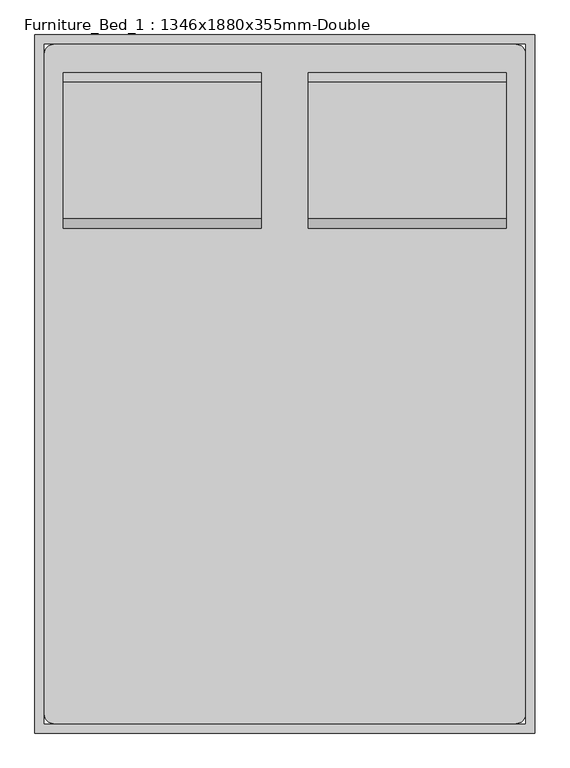
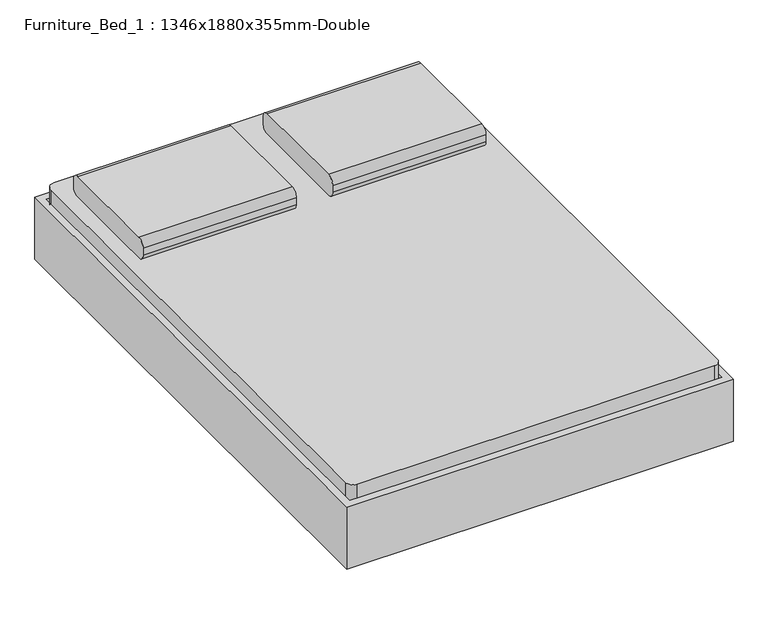
"""IFC4 building model written with IfcOpenShell, lengths in millimetres: furniture geometry, Furniture_Bed_1 : 1346x1880x355mm-Double."""

from ifc_helpers import new_model, si_unit, point, frame, frame_2d, origin, place, context, project, spatial, polyline, circle_curve, trimmed, segment, composite_curve, outline, extrude, source, transform, mapped, element, save
from ifc_brep_helpers import plane_surface, cylinder_surface, revolved_surface, advanced_brep


def furniture_bed_1_1346x1880x355mm_double_93dec6ea(model_context):
    return source(origin(), model_context, "Body", "SolidModel", [
        advanced_brep(
        [(-308.447541, -869.6295082, 196.85), (-308.447541, -869.6295082, 177.8), (-308.447541, -945.8295082, 177.8), (-308.447541, -945.8295082, 196.85), (-245.5113525, -869.6295082, 196.85), (-257.647541, -869.6295082, 177.8), (-257.647541, -945.8295082, 177.8), (-245.5113525, -945.8295082, 196.85), (-164.3115092, -869.6295082, 22.716374), (-181.5766725, -869.6295082, 14.6654962), (-181.5766725, -945.8295082, 14.6654962), (-164.3115092, -945.8295082, 22.716374), (-158.5564547, -869.6295082, 0.0), (-158.5564547, -869.6295082, 19.05), (-158.5564547, -945.8295082, 0.0), (-158.5564547, -945.8295082, 19.05), (-79.9439489, -869.6295082, 19.05), (-79.9439489, -869.6295082, 0.0), (-79.9439489, -945.8295082, 0.0), (-79.9439489, -945.8295082, 19.05), (-67.2439489, -869.6295082, 3.4029547), (-76.7689489, -869.6295082, 19.9007387), (-67.2439489, -945.8295082, 3.4029547), (-76.7689489, -945.8295082, 19.9007387), (-12.2513357, -869.6295082, 57.15), (-7.1469036, -869.6295082, 38.1), (-7.1469036, -945.8295082, 38.1), (-12.2513357, -945.8295082, 57.15), (690.5562537, -869.6295082, 57.15), (685.4518216, -869.6295082, 38.1), (685.4518216, -945.8295082, 38.1), (690.5562537, -945.8295082, 57.15), (755.0738669, -869.6295082, 19.9007387), (745.5488669, -869.6295082, 3.4029547), (745.5488669, -945.8295082, 3.4029547), (755.0738669, -945.8295082, 19.9007387), (758.2488669, -869.6295082, 0.0), (758.2488669, -869.6295082, 19.05), (758.2488669, -945.8295082, 0.0), (758.2488669, -945.8295082, 19.05), (836.8613728, -869.6295082, 19.05), (836.8613728, -869.6295082, 0.0), (836.8613728, -945.8295082, 0.0), (836.8613728, -945.8295082, 19.05), (859.8815906, -869.6295082, 14.6654962), (842.6164272, -869.6295082, 22.716374), (859.8815906, -945.8295082, 14.6654962), (842.6164272, -945.8295082, 22.716374), (923.8162705, -869.6295082, 196.85), (935.952459, -869.6295082, 177.8), (935.952459, -945.8295082, 177.8), (923.8162705, -945.8295082, 196.85), (986.752459, -869.6295082, 196.85), (986.752459, -945.8295082, 196.85), (986.752459, -945.8295082, 177.8), (986.752459, -869.6295082, 177.8)],
        [
            (0, 1),
            (1, 2),
            (2, 3),
            (3, 0),
            (0, 4),
            (4, 5),
            (5, 1),
            (5, 6),
            (6, 2),
            (6, 7),
            (7, 3),
            (7, 4),
            (4, 8),
            (8, 9),
            (9, 5),
            (9, 10),
            (10, 6),
            (10, 11),
            (11, 7),
            (11, 8),
            (12, 9, circle_curve(frame((-158.5564547, -869.6295082, 25.4), z_axis=(0.0, 1.0, 0.0), x_axis=(-0.9063077870366627, 0.0, -0.42261826174067213)), 25.4)),
            (8, 13, circle_curve(frame((-158.5564547, -869.6295082, 25.4), z_axis=(0.0, -1.0, 0.0), x_axis=(-0.9063077870366627, 0.0, -0.42261826174067213)), 6.35)),
            (13, 12),
            (14, 10, circle_curve(frame((-158.5564547, -945.8295082, 25.4), z_axis=(0.0, 1.0, 0.0), x_axis=(-0.9063077870366627, 0.0, -0.42261826174067213)), 25.4)),
            (12, 14),
            (15, 11, circle_curve(frame((-158.5564547, -945.8295082, 25.4), z_axis=(0.0, 1.0, 0.0), x_axis=(-0.9063077870366627, 0.0, -0.42261826174067213)), 6.35)),
            (14, 15),
            (15, 13),
            (13, 16),
            (16, 17),
            (17, 12),
            (17, 18),
            (18, 14),
            (18, 19),
            (19, 15),
            (19, 16),
            (20, 17, circle_curve(frame((-79.9439489, -869.6295082, 25.4), z_axis=(0.0, 1.0, 0.0), x_axis=(0.0, 0.0, -1.0)), 25.4)),
            (16, 21, circle_curve(frame((-79.9439489, -869.6295082, 25.4), z_axis=(0.0, -1.0, 0.0), x_axis=(0.0, 0.0, -1.0)), 6.35)),
            (21, 20),
            (22, 18, circle_curve(frame((-79.9439489, -945.8295082, 25.4), z_axis=(0.0, 1.0, 0.0), x_axis=(0.0, 0.0, -1.0)), 25.4)),
            (20, 22),
            (23, 19, circle_curve(frame((-79.9439489, -945.8295082, 25.4), z_axis=(0.0, 1.0, 0.0), x_axis=(0.0, 0.0, -1.0)), 6.35)),
            (22, 23),
            (23, 21),
            (21, 24),
            (24, 25),
            (25, 20),
            (25, 26),
            (26, 22),
            (26, 27),
            (27, 23),
            (27, 24),
            (24, 28),
            (28, 29),
            (29, 25),
            (29, 30),
            (30, 26),
            (30, 31),
            (31, 27),
            (31, 28),
            (28, 32),
            (32, 33),
            (33, 29),
            (33, 34),
            (34, 30),
            (34, 35),
            (35, 31),
            (35, 32),
            (36, 33, circle_curve(frame((758.2488669, -869.6295082, 25.4), z_axis=(0.0, 1.0, 0.0), x_axis=(-0.5000000000000486, 0.0, -0.8660254037844105)), 25.4)),
            (32, 37, circle_curve(frame((758.2488669, -869.6295082, 25.4), z_axis=(0.0, -1.0, 0.0), x_axis=(-0.5000000000000486, 0.0, -0.8660254037844105)), 6.35)),
            (37, 36),
            (38, 34, circle_curve(frame((758.2488669, -945.8295082, 25.4), z_axis=(0.0, 1.0, 0.0), x_axis=(-0.5000000000000486, 0.0, -0.8660254037844105)), 25.4)),
            (36, 38),
            (39, 35, circle_curve(frame((758.2488669, -945.8295082, 25.4), z_axis=(0.0, 1.0, 0.0), x_axis=(-0.5000000000000486, 0.0, -0.8660254037844105)), 6.35)),
            (38, 39),
            (39, 37),
            (37, 40),
            (40, 41),
            (41, 36),
            (41, 42),
            (42, 38),
            (42, 43),
            (43, 39),
            (43, 40),
            (44, 41, circle_curve(frame((836.8613728, -869.6295082, 25.4), z_axis=(0.0, 1.0, 0.0), x_axis=(0.0, 0.0, -1.0)), 25.4)),
            (40, 45, circle_curve(frame((836.8613728, -869.6295082, 25.4), z_axis=(0.0, -1.0, 0.0), x_axis=(0.0, 0.0, -1.0)), 6.35)),
            (45, 44),
            (46, 42, circle_curve(frame((836.8613728, -945.8295082, 25.4), z_axis=(0.0, 1.0, 0.0), x_axis=(0.0, 0.0, -1.0)), 25.4)),
            (44, 46),
            (47, 43, circle_curve(frame((836.8613728, -945.8295082, 25.4), z_axis=(0.0, 1.0, 0.0), x_axis=(0.0, 0.0, -1.0)), 6.35)),
            (46, 47),
            (47, 45),
            (45, 48),
            (48, 49),
            (49, 44),
            (49, 50),
            (50, 46),
            (50, 51),
            (51, 47),
            (51, 48),
            (52, 53),
            (53, 54),
            (54, 55),
            (55, 52),
            (48, 52),
            (55, 49),
            (54, 50),
            (53, 51),
        ],
        [
            plane_surface(frame((-308.447541, -1174.4295082, -127.5947323), z_axis=(-1.0, 0.0, 0.0), x_axis=(0.0, 1.0, 0.0))),
            plane_surface(frame((-308.447541, -869.6295082, 196.85), z_axis=(0.0, 1.0, 0.0), x_axis=(1.0, 0.0, 0.0))),
            plane_surface(frame((-308.447541, -869.6295082, 177.8), z_axis=(0.0, 0.0, -1.0), x_axis=(1.0, 0.0, 0.0))),
            plane_surface(frame((-308.447541, -945.8295082, 177.8), z_axis=(0.0, -1.0, 0.0), x_axis=(1.0, 0.0, 0.0))),
            plane_surface(frame((-308.447541, -945.8295082, 196.85), z_axis=(0.0, 0.0, 1.0), x_axis=(1.0, 0.0, 0.0))),
            plane_surface(frame((-245.5113525, -869.6295082, 196.85), z_axis=(0.0, 1.0, 0.0), x_axis=(0.42261826174067146, 0.0, -0.906307787036663))),
            plane_surface(frame((-257.647541, -869.6295082, 177.8), z_axis=(-0.9063077870366631, 0.0, -0.4226182617406713), x_axis=(0.4226182617406713, 0.0, -0.9063077870366631))),
            plane_surface(frame((-257.647541, -945.8295082, 177.8), z_axis=(0.0, -1.0, 0.0), x_axis=(0.4226182617406716, 0.0, -0.9063077870366629))),
            plane_surface(frame((-245.5113525, -945.8295082, 196.85), z_axis=(0.906307787036663, 0.0, 0.4226182617406716), x_axis=(0.4226182617406716, 0.0, -0.906307787036663))),
            plane_surface(frame((-158.5564547, -869.6295082, 25.4), z_axis=(0.0, 1.0, 0.0), x_axis=(-0.9063077870366627, 0.0, -0.42261826174067213))),
            cylinder_surface(frame((-158.5564547, -1174.4295082, 25.4), z_axis=(0.0, -1.0, 0.0), x_axis=(-0.9063077870366627, 0.0, -0.42261826174067213)), 25.4),
            plane_surface(frame((-158.5564547, -945.8295082, 25.4), z_axis=(0.0, -1.0, 0.0), x_axis=(-0.9063077870366627, 0.0, -0.42261826174067213))),
            revolved_surface(polyline([(-164.31150914768278, -945.8295082, 22.716374037946732), (-164.31150914768278, -869.6295082, 22.716374037946732)]), (-158.5564547, -1174.4295082, 25.4), (0.0, -1.0, 0.0)),
            plane_surface(frame((-158.5564547, -869.6295082, 19.05), z_axis=(0.0, 1.0, 0.0), x_axis=(1.0, 0.0, 0.0))),
            plane_surface(frame((-158.5564547, -869.6295082, 0.0), z_axis=(0.0, 0.0, -1.0), x_axis=(1.0, 0.0, 0.0))),
            plane_surface(frame((-158.5564547, -945.8295082, 0.0), z_axis=(0.0, -1.0, 0.0), x_axis=(1.0, 0.0, 0.0))),
            plane_surface(frame((-158.5564547, -945.8295082, 19.05), z_axis=(0.0, 0.0, 1.0), x_axis=(1.0, 0.0, 0.0))),
            plane_surface(frame((-79.9439489, -869.6295082, 25.4), z_axis=(0.0, 1.0, 0.0), x_axis=(0.0, 0.0, -1.0))),
            cylinder_surface(frame((-79.9439489, -1174.4295082, 25.4), z_axis=(0.0, -1.0, 0.0), x_axis=(0.0, 0.0, -1.0)), 25.4),
            plane_surface(frame((-79.9439489, -945.8295082, 25.4), z_axis=(0.0, -1.0, 0.0), x_axis=(0.0, 0.0, -1.0))),
            revolved_surface(polyline([(-79.9439489, -945.8295082, 19.049999999999997), (-79.9439489, -869.6295082, 19.049999999999997)]), (-79.9439489, -1174.4295082, 25.4), (0.0, -1.0, 0.0)),
            plane_surface(frame((-76.7689489, -869.6295082, 19.9007387), z_axis=(0.0, 1.0, 0.0), x_axis=(0.8660254037844782, 0.0, 0.4999999999999314))),
            plane_surface(frame((-67.2439489, -869.6295082, 3.4029547), z_axis=(0.49999999999993133, 0.0, -0.8660254037844783), x_axis=(0.8660254037844783, 0.0, 0.49999999999993133))),
            plane_surface(frame((-67.2439489, -945.8295082, 3.4029547), z_axis=(0.0, -1.0, 0.0), x_axis=(0.8660254037844785, 0.0, 0.499999999999931))),
            plane_surface(frame((-76.7689489, -945.8295082, 19.9007387), z_axis=(-0.49999999999993144, 0.0, 0.8660254037844782), x_axis=(0.8660254037844782, 0.0, 0.49999999999993144))),
            plane_surface(frame((-12.2513357, -869.6295082, 57.15), z_axis=(0.0, 1.0, 0.0), x_axis=(1.0, 0.0, 0.0))),
            plane_surface(frame((-7.1469036, -869.6295082, 38.1), z_axis=(0.0, 0.0, -1.0), x_axis=(1.0, 0.0, 0.0))),
            plane_surface(frame((-7.1469036, -945.8295082, 38.1), z_axis=(0.0, -1.0, 0.0), x_axis=(1.0, 0.0, 0.0))),
            plane_surface(frame((-12.2513357, -945.8295082, 57.15), z_axis=(0.0, 0.0, 1.0), x_axis=(1.0, 0.0, 0.0))),
            plane_surface(frame((690.5562537, -869.6295082, 57.15), z_axis=(0.0, 1.0, 0.0), x_axis=(0.8660254037844104, 0.0, -0.5000000000000491))),
            plane_surface(frame((685.4518216, -869.6295082, 38.1), z_axis=(-0.5000000000000484, 0.0, -0.8660254037844108), x_axis=(0.8660254037844108, 0.0, -0.5000000000000484))),
            plane_surface(frame((685.4518216, -945.8295082, 38.1), z_axis=(0.0, -1.0000000000000002, 0.0), x_axis=(0.8660254037844103, 0.0, -0.5000000000000493))),
            plane_surface(frame((690.5562537, -945.8295082, 57.15), z_axis=(0.5000000000000485, 0.0, 0.8660254037844106), x_axis=(0.8660254037844106, 0.0, -0.5000000000000485))),
            plane_surface(frame((758.2488669, -869.6295082, 25.4), z_axis=(0.0, 1.0000000000000002, 0.0), x_axis=(-0.5000000000000487, 0.0, -0.8660254037844106))),
            cylinder_surface(frame((758.2488669, -1174.4295082, 25.4), z_axis=(0.0, -1.0, 0.0), x_axis=(-0.5000000000000486, 0.0, -0.8660254037844105)), 25.4),
            plane_surface(frame((758.2488669, -945.8295082, 25.4), z_axis=(0.0, -1.0000000000000002, 0.0), x_axis=(-0.5000000000000487, 0.0, -0.8660254037844106))),
            revolved_surface(polyline([(755.0738668999998, -945.8295082, 19.900738685968992), (755.0738668999998, -869.6295082, 19.900738685968992)]), (758.2488669, -1174.4295082, 25.4), (0.0, -1.0, 0.0)),
            plane_surface(frame((758.2488669, -869.6295082, 19.05), z_axis=(0.0, 1.0, 0.0), x_axis=(1.0, 0.0, 0.0))),
            plane_surface(frame((758.2488669, -869.6295082, 0.0), z_axis=(0.0, 0.0, -1.0), x_axis=(1.0, 0.0, 0.0))),
            plane_surface(frame((758.2488669, -945.8295082, 0.0), z_axis=(0.0, -1.0, 0.0), x_axis=(1.0, 0.0, 0.0))),
            plane_surface(frame((758.2488669, -945.8295082, 19.05), z_axis=(0.0, 0.0, 1.0), x_axis=(1.0, 0.0, 0.0))),
            plane_surface(frame((836.8613728, -869.6295082, 25.4), z_axis=(0.0, 1.0, 0.0), x_axis=(0.0, 0.0, -1.0))),
            cylinder_surface(frame((836.8613728, -1174.4295082, 25.4), z_axis=(0.0, -1.0, 0.0), x_axis=(0.0, 0.0, -1.0)), 25.4),
            plane_surface(frame((836.8613728, -945.8295082, 25.4), z_axis=(0.0, -1.0, 0.0), x_axis=(0.0, 0.0, -1.0))),
            revolved_surface(polyline([(836.8613728, -945.8295082, 19.049999999999997), (836.8613728, -869.6295082, 19.049999999999997)]), (836.8613728, -1174.4295082, 25.4), (0.0, -1.0, 0.0)),
            plane_surface(frame((842.6164272, -869.6295082, 22.716374), z_axis=(0.0, 1.0, 0.0), x_axis=(0.4226182617405402, 0.0, 0.9063077870367242))),
            plane_surface(frame((859.8815906, -869.6295082, 14.6654962), z_axis=(0.9063077870367245, 0.0, -0.42261826174053974), x_axis=(0.42261826174053974, 0.0, 0.9063077870367245))),
            plane_surface(frame((859.8815906, -945.8295082, 14.6654962), z_axis=(0.0, -1.0000000000000002, 0.0), x_axis=(0.42261826174053974, 0.0, 0.9063077870367245))),
            plane_surface(frame((842.6164272, -945.8295082, 22.716374), z_axis=(-0.9063077870367247, 0.0, 0.4226182617405394), x_axis=(0.4226182617405394, 0.0, 0.9063077870367247))),
            plane_surface(frame((986.752459, -1174.4295082, -127.5947323), z_axis=(1.0, 0.0, 0.0), x_axis=(0.0, 1.0, 0.0))),
            plane_surface(frame((923.8162705, -869.6295082, 196.85), z_axis=(0.0, 1.0, 0.0), x_axis=(1.0, 0.0, 0.0))),
            plane_surface(frame((935.952459, -869.6295082, 177.8), z_axis=(0.0, 0.0, -1.0), x_axis=(1.0, 0.0, 0.0))),
            plane_surface(frame((935.952459, -945.8295082, 177.8), z_axis=(0.0, -1.0, 0.0), x_axis=(1.0, 0.0, 0.0))),
            plane_surface(frame((923.8162705, -945.8295082, 196.85), z_axis=(0.0, 0.0, 1.0), x_axis=(1.0, 0.0, 0.0))),
        ],
        [
            (0, [[1, 2, 3, 4]]),
            (1, [[-1, 5, 6, 7]]),
            (2, [[-2, -7, 8, 9]]),
            (3, [[-3, -9, 10, 11]]),
            (4, [[-4, -11, 12, -5]]),
            (5, [[-6, 13, 14, 15]]),
            (6, [[-8, -15, 16, 17]]),
            (7, [[-10, -17, 18, 19]]),
            (8, [[-12, -19, 20, -13]]),
            (9, [[21, -14, 22, 23]]),
            (10, [[24, -16, -21, 25]]),
            (11, [[26, -18, -24, 27]]),
            (12, [[-22, -20, -26, 28]]),
            (13, [[-23, 29, 30, 31]]),
            (14, [[-25, -31, 32, 33]]),
            (15, [[-27, -33, 34, 35]]),
            (16, [[-28, -35, 36, -29]]),
            (17, [[37, -30, 38, 39]]),
            (18, [[40, -32, -37, 41]]),
            (19, [[42, -34, -40, 43]]),
            (20, [[-38, -36, -42, 44]]),
            (21, [[-39, 45, 46, 47]]),
            (22, [[-41, -47, 48, 49]]),
            (23, [[-43, -49, 50, 51]]),
            (24, [[-44, -51, 52, -45]]),
            (25, [[-46, 53, 54, 55]]),
            (26, [[-48, -55, 56, 57]]),
            (27, [[-50, -57, 58, 59]]),
            (28, [[-52, -59, 60, -53]]),
            (29, [[-54, 61, 62, 63]]),
            (30, [[-56, -63, 64, 65]]),
            (31, [[-58, -65, 66, 67]]),
            (32, [[-60, -67, 68, -61]]),
            (33, [[69, -62, 70, 71]]),
            (34, [[72, -64, -69, 73]]),
            (35, [[74, -66, -72, 75]]),
            (36, [[-70, -68, -74, 76]]),
            (37, [[-71, 77, 78, 79]]),
            (38, [[-73, -79, 80, 81]]),
            (39, [[-75, -81, 82, 83]]),
            (40, [[-76, -83, 84, -77]]),
            (41, [[85, -78, 86, 87]]),
            (42, [[88, -80, -85, 89]]),
            (43, [[90, -82, -88, 91]]),
            (44, [[-86, -84, -90, 92]]),
            (45, [[-87, 93, 94, 95]]),
            (46, [[-89, -95, 96, 97]]),
            (47, [[-91, -97, 98, 99]]),
            (48, [[-92, -99, 100, -93]]),
            (49, [[101, 102, 103, 104]]),
            (50, [[-94, 105, -104, 106]]),
            (51, [[-96, -106, -103, 107]]),
            (52, [[-98, -107, -102, 108]]),
            (53, [[-100, -108, -101, -105]]),
        ],
    ),
        extrude(outline(composite_curve([segment(polyline([(-283.047541, 680.1704918), (961.352459, 680.1704918)]), True, "CONTINUOUS"), segment(trimmed(circle_curve(frame_2d((961.352459, 654.7704918)), 25.4), [point((961.352459, 680.1704918))], [point((986.752459, 654.7704918))], False, "CARTESIAN"), True, "CONTINUOUS"), segment(polyline([(986.752459, 654.7704918), (986.752459, -1123.6295082)]), True, "CONTINUOUS"), segment(trimmed(circle_curve(frame_2d((961.352459, -1123.6295082)), 25.4), [point((986.752459, -1123.6295082))], [point((961.352459, -1149.0295082))], False, "CARTESIAN"), True, "CONTINUOUS"), segment(polyline([(961.352459, -1149.0295082), (-283.047541, -1149.0295082)]), True, "CONTINUOUS"), segment(trimmed(circle_curve(frame_2d((-283.047541, -1123.6295082)), 25.4), [point((-283.047541, -1149.0295082))], [point((-308.447541, -1123.6295082))], False, "CARTESIAN"), True, "CONTINUOUS"), segment(polyline([(-308.447541, -1123.6295082), (-308.447541, 654.7704918)]), True, "CONTINUOUS"), segment(trimmed(circle_curve(frame_2d((-283.047541, 654.7704918)), 25.4), [point((-308.447541, 654.7704918))], [point((-283.047541, 680.1704918))], False, "CARTESIAN"), True, "CONTINUOUS")], self_intersect=False)), frame((0.0, 0.0, 203.2), z_axis=(0.0, 0.0, 1.0), x_axis=(1.0, 0.0, 0.0)), (0.0, 0.0, 1.0), 203.2),
        advanced_brep(
        [(-308.1231784, 451.5704918, 177.8), (-308.1231784, 375.3704918, 177.8), (-308.1231784, 375.3704918, 196.85), (-308.1231784, 451.5704918, 196.85), (-257.3231784, 451.5704918, 177.8), (-257.3231784, 375.3704918, 177.8), (-245.1869899, 375.3704918, 196.85), (-245.1869899, 451.5704918, 196.85), (-181.2523099, 451.5704918, 14.6654962), (-181.2523099, 375.3704918, 14.6654962), (-163.9871466, 375.3704918, 22.716374), (-163.9871466, 451.5704918, 22.716374), (-158.2320921, 375.3704918, 0.0), (-158.2320921, 451.5704918, 0.0), (-158.2320921, 375.3704918, 19.05), (-158.2320921, 451.5704918, 19.05), (-79.6195862, 451.5704918, 0.0), (-79.6195862, 375.3704918, 0.0), (-79.6195862, 375.3704918, 19.05), (-79.6195862, 451.5704918, 19.05), (-66.9195862, 375.3704918, 3.4029547), (-66.9195862, 451.5704918, 3.4029547), (-76.4445862, 375.3704918, 19.9007387), (-76.4445862, 451.5704918, 19.9007387), (-6.822541, 451.5704918, 38.1), (-6.822541, 375.3704918, 38.1), (-11.9269731, 375.3704918, 57.15), (-11.9269731, 451.5704918, 57.15), (685.4518216, 451.5704918, 38.1), (685.4518216, 375.3704918, 38.1), (690.5562537, 375.3704918, 57.15), (690.5562537, 451.5704918, 57.15), (745.5488669, 451.5704918, 3.4029547), (745.5488669, 375.3704918, 3.4029547), (755.0738669, 375.3704918, 19.9007387), (755.0738669, 451.5704918, 19.9007387), (758.2488669, 375.3704918, 0.0), (758.2488669, 451.5704918, 0.0), (758.2488669, 375.3704918, 19.05), (758.2488669, 451.5704918, 19.05), (836.8613728, 451.5704918, 0.0), (836.8613728, 375.3704918, 0.0), (836.8613728, 375.3704918, 19.05), (836.8613728, 451.5704918, 19.05), (859.8815906, 375.3704918, 14.6654962), (859.8815906, 451.5704918, 14.6654962), (842.6164272, 375.3704918, 22.716374), (842.6164272, 451.5704918, 22.716374), (935.952459, 451.5704918, 177.8), (935.952459, 375.3704918, 177.8), (923.8162705, 375.3704918, 196.85), (923.8162705, 451.5704918, 196.85), (986.752459, 451.5704918, 177.8), (986.752459, 451.5704918, 196.85), (986.752459, 375.3704918, 196.85), (986.752459, 375.3704918, 177.8)],
        [
            (0, 1),
            (1, 2),
            (2, 3),
            (3, 0),
            (0, 4),
            (4, 5),
            (5, 1),
            (5, 6),
            (6, 2),
            (6, 7),
            (7, 3),
            (7, 4),
            (4, 8),
            (8, 9),
            (9, 5),
            (9, 10),
            (10, 6),
            (10, 11),
            (11, 7),
            (11, 8),
            (12, 9, circle_curve(frame((-158.2320921, 375.3704918, 25.4), z_axis=(0.0, 1.0, 0.0), x_axis=(-0.906307787036649, 0.0, -0.4226182617407015)), 25.4)),
            (8, 13, circle_curve(frame((-158.2320921, 451.5704918, 25.4), z_axis=(0.0, -1.0, 0.0), x_axis=(-0.906307787036649, 0.0, -0.4226182617407015)), 25.4)),
            (13, 12),
            (14, 10, circle_curve(frame((-158.2320921, 375.3704918, 25.4), z_axis=(0.0, 1.0, 0.0), x_axis=(-0.906307787036649, 0.0, -0.4226182617407015)), 6.35)),
            (12, 14),
            (15, 11, circle_curve(frame((-158.2320921, 451.5704918, 25.4), z_axis=(0.0, 1.0, 0.0), x_axis=(-0.906307787036649, 0.0, -0.4226182617407015)), 6.35)),
            (14, 15),
            (15, 13),
            (13, 16),
            (16, 17),
            (17, 12),
            (17, 18),
            (18, 14),
            (18, 19),
            (19, 15),
            (19, 16),
            (20, 17, circle_curve(frame((-79.6195862, 375.3704918, 25.4), z_axis=(0.0, 1.0, 0.0), x_axis=(0.0, 0.0, -1.0)), 25.4)),
            (16, 21, circle_curve(frame((-79.6195862, 451.5704918, 25.4), z_axis=(0.0, -1.0, 0.0), x_axis=(0.0, 0.0, -1.0)), 25.4)),
            (21, 20),
            (22, 18, circle_curve(frame((-79.6195862, 375.3704918, 25.4), z_axis=(0.0, 1.0, 0.0), x_axis=(0.0, 0.0, -1.0)), 6.35)),
            (20, 22),
            (23, 19, circle_curve(frame((-79.6195862, 451.5704918, 25.4), z_axis=(0.0, 1.0, 0.0), x_axis=(0.0, 0.0, -1.0)), 6.35)),
            (22, 23),
            (23, 21),
            (21, 24),
            (24, 25),
            (25, 20),
            (25, 26),
            (26, 22),
            (26, 27),
            (27, 23),
            (27, 24),
            (24, 28),
            (28, 29),
            (29, 25),
            (29, 30),
            (30, 26),
            (30, 31),
            (31, 27),
            (31, 28),
            (28, 32),
            (32, 33),
            (33, 29),
            (33, 34),
            (34, 30),
            (34, 35),
            (35, 31),
            (35, 32),
            (36, 33, circle_curve(frame((758.2488669, 375.3704918, 25.4), z_axis=(0.0, 1.0, 0.0), x_axis=(-0.5000000000000444, 0.0, -0.866025403784413)), 25.4)),
            (32, 37, circle_curve(frame((758.2488669, 451.5704918, 25.4), z_axis=(0.0, -1.0, 0.0), x_axis=(-0.5000000000000444, 0.0, -0.866025403784413)), 25.4)),
            (37, 36),
            (38, 34, circle_curve(frame((758.2488669, 375.3704918, 25.4), z_axis=(0.0, 1.0, 0.0), x_axis=(-0.5000000000000444, 0.0, -0.866025403784413)), 6.35)),
            (36, 38),
            (39, 35, circle_curve(frame((758.2488669, 451.5704918, 25.4), z_axis=(0.0, 1.0, 0.0), x_axis=(-0.5000000000000444, 0.0, -0.866025403784413)), 6.35)),
            (38, 39),
            (39, 37),
            (37, 40),
            (40, 41),
            (41, 36),
            (41, 42),
            (42, 38),
            (42, 43),
            (43, 39),
            (43, 40),
            (44, 41, circle_curve(frame((836.8613728, 375.3704918, 25.4), z_axis=(0.0, 1.0, 0.0), x_axis=(0.0, 0.0, -1.0)), 25.4)),
            (40, 45, circle_curve(frame((836.8613728, 451.5704918, 25.4), z_axis=(0.0, -1.0, 0.0), x_axis=(0.0, 0.0, -1.0)), 25.4)),
            (45, 44),
            (46, 42, circle_curve(frame((836.8613728, 375.3704918, 25.4), z_axis=(0.0, 1.0, 0.0), x_axis=(0.0, 0.0, -1.0)), 6.35)),
            (44, 46),
            (47, 43, circle_curve(frame((836.8613728, 451.5704918, 25.4), z_axis=(0.0, 1.0, 0.0), x_axis=(0.0, 0.0, -1.0)), 6.35)),
            (46, 47),
            (47, 45),
            (45, 48),
            (48, 49),
            (49, 44),
            (49, 50),
            (50, 46),
            (50, 51),
            (51, 47),
            (51, 48),
            (52, 53),
            (53, 54),
            (54, 55),
            (55, 52),
            (48, 52),
            (55, 49),
            (54, 50),
            (53, 51),
        ],
        [
            plane_surface(frame((-308.1231784, 705.5704918, -152.9490627), z_axis=(-1.0, 0.0, 0.0), x_axis=(0.0, 1.0, 0.0))),
            plane_surface(frame((-308.1231784, 451.5704918, 177.8), z_axis=(0.0, 0.0, -1.0), x_axis=(1.0, 0.0, 0.0))),
            plane_surface(frame((-308.1231784, 375.3704918, 177.8), z_axis=(0.0, -1.0, 0.0), x_axis=(1.0, 0.0, 0.0))),
            plane_surface(frame((-308.1231784, 375.3704918, 196.85), z_axis=(0.0, 0.0, 1.0), x_axis=(1.0, 0.0, 0.0))),
            plane_surface(frame((-308.1231784, 451.5704918, 196.85), z_axis=(0.0, 1.0, 0.0), x_axis=(1.0, 0.0, 0.0))),
            plane_surface(frame((-257.3231784, 451.5704918, 177.8), z_axis=(-0.9063077870366483, 0.0, -0.4226182617407031), x_axis=(0.4226182617407031, 0.0, -0.9063077870366483))),
            plane_surface(frame((-257.3231784, 375.3704918, 177.8), z_axis=(0.0, -1.0, 0.0), x_axis=(0.4226182617407027, 0.0, -0.9063077870366485))),
            plane_surface(frame((-245.1869899, 375.3704918, 196.85), z_axis=(0.9063077870366484, 0.0, 0.4226182617407029), x_axis=(0.4226182617407029, 0.0, -0.9063077870366484))),
            plane_surface(frame((-245.1869899, 451.5704918, 196.85), z_axis=(0.0, 1.0, 0.0), x_axis=(0.4226182617407027, 0.0, -0.9063077870366485))),
            cylinder_surface(frame((-158.2320921, 705.5704918, 25.4), z_axis=(0.0, -1.0, 0.0), x_axis=(-0.906307787036649, 0.0, -0.4226182617407015)), 25.4),
            plane_surface(frame((-158.2320921, 375.3704918, 25.4), z_axis=(0.0, -1.0, 0.0), x_axis=(-0.906307787036649, 0.0, -0.4226182617407015))),
            revolved_surface(polyline([(-163.9871465476827, 375.3704918, 22.716374037946544), (-163.9871465476827, 451.5704918, 22.716374037946544)]), (-158.2320921, 705.5704918, 25.4), (0.0, -1.0, 0.0)),
            plane_surface(frame((-158.2320921, 451.5704918, 25.4), z_axis=(0.0, 1.0, 0.0), x_axis=(-0.906307787036649, 0.0, -0.4226182617407015))),
            plane_surface(frame((-158.2320921, 451.5704918, 0.0), z_axis=(0.0, 0.0, -1.0), x_axis=(1.0, 0.0, 0.0))),
            plane_surface(frame((-158.2320921, 375.3704918, 0.0), z_axis=(0.0, -1.0, 0.0), x_axis=(1.0, 0.0, 0.0))),
            plane_surface(frame((-158.2320921, 375.3704918, 19.05), z_axis=(0.0, 0.0, 1.0), x_axis=(1.0, 0.0, 0.0))),
            plane_surface(frame((-158.2320921, 451.5704918, 19.05), z_axis=(0.0, 1.0, 0.0), x_axis=(1.0, 0.0, 0.0))),
            cylinder_surface(frame((-79.6195862, 705.5704918, 25.4), z_axis=(0.0, -1.0, 0.0), x_axis=(0.0, 0.0, -1.0)), 25.4),
            plane_surface(frame((-79.6195862, 375.3704918, 25.4), z_axis=(0.0, -1.0, 0.0), x_axis=(0.0, 0.0, -1.0))),
            revolved_surface(polyline([(-79.6195862, 375.3704918, 19.049999999999997), (-79.6195862, 451.5704918, 19.049999999999997)]), (-79.6195862, 705.5704918, 25.4), (0.0, -1.0, 0.0)),
            plane_surface(frame((-79.6195862, 451.5704918, 25.4), z_axis=(0.0, 1.0, 0.0), x_axis=(0.0, 0.0, -1.0))),
            plane_surface(frame((-66.9195862, 451.5704918, 3.4029547), z_axis=(0.4999999999998771, 0.0, -0.8660254037845097), x_axis=(0.8660254037845097, 0.0, 0.4999999999998771))),
            plane_surface(frame((-66.9195862, 375.3704918, 3.4029547), z_axis=(0.0, -1.0000000000000002, 0.0), x_axis=(0.8660254037845102, 0.0, 0.49999999999987627))),
            plane_surface(frame((-76.4445862, 375.3704918, 19.9007387), z_axis=(-0.49999999999987643, 0.0, 0.86602540378451), x_axis=(0.86602540378451, 0.0, 0.49999999999987643))),
            plane_surface(frame((-76.4445862, 451.5704918, 19.9007387), z_axis=(0.0, 1.0, 0.0), x_axis=(0.8660254037845102, 0.0, 0.4999999999998761))),
            plane_surface(frame((-6.822541, 451.5704918, 38.1), z_axis=(0.0, 0.0, -1.0), x_axis=(1.0, 0.0, 0.0))),
            plane_surface(frame((-6.822541, 375.3704918, 38.1), z_axis=(0.0, -1.0, 0.0), x_axis=(1.0, 0.0, 0.0))),
            plane_surface(frame((-11.9269731, 375.3704918, 57.15), z_axis=(0.0, 0.0, 1.0), x_axis=(1.0, 0.0, 0.0))),
            plane_surface(frame((-11.9269731, 451.5704918, 57.15), z_axis=(0.0, 1.0, 0.0), x_axis=(1.0, 0.0, 0.0))),
            plane_surface(frame((685.4518216, 451.5704918, 38.1), z_axis=(-0.5000000000000445, 0.0, -0.866025403784413), x_axis=(0.866025403784413, 0.0, -0.5000000000000445))),
            plane_surface(frame((685.4518216, 375.3704918, 38.1), z_axis=(0.0, -1.0, 0.0), x_axis=(0.8660254037844118, 0.0, -0.5000000000000464))),
            plane_surface(frame((690.5562537, 375.3704918, 57.15), z_axis=(0.5000000000000461, 0.0, 0.8660254037844121), x_axis=(0.8660254037844121, 0.0, -0.5000000000000461))),
            plane_surface(frame((690.5562537, 451.5704918, 57.15), z_axis=(0.0, 1.0, 0.0), x_axis=(0.8660254037844126, 0.0, -0.5000000000000452))),
            cylinder_surface(frame((758.2488669, 705.5704918, 25.4), z_axis=(0.0, -1.0, 0.0), x_axis=(-0.5000000000000444, 0.0, -0.866025403784413)), 25.4),
            plane_surface(frame((758.2488669, 375.3704918, 25.4), z_axis=(0.0, -1.0000000000000002, 0.0), x_axis=(-0.5000000000000445, 0.0, -0.8660254037844131))),
            revolved_surface(polyline([(755.0738668999998, 375.3704918, 19.900738685968975), (755.0738668999998, 451.5704918, 19.900738685968975)]), (758.2488669, 705.5704918, 25.4), (0.0, -1.0, 0.0)),
            plane_surface(frame((758.2488669, 451.5704918, 25.4), z_axis=(0.0, 1.0000000000000002, 0.0), x_axis=(-0.5000000000000445, 0.0, -0.8660254037844131))),
            plane_surface(frame((758.2488669, 451.5704918, 0.0), z_axis=(0.0, 0.0, -1.0), x_axis=(1.0, 0.0, 0.0))),
            plane_surface(frame((758.2488669, 375.3704918, 0.0), z_axis=(0.0, -1.0, 0.0), x_axis=(1.0, 0.0, 0.0))),
            plane_surface(frame((758.2488669, 375.3704918, 19.05), z_axis=(0.0, 0.0, 1.0), x_axis=(1.0, 0.0, 0.0))),
            plane_surface(frame((758.2488669, 451.5704918, 19.05), z_axis=(0.0, 1.0, 0.0), x_axis=(1.0, 0.0, 0.0))),
            cylinder_surface(frame((836.8613728, 705.5704918, 25.4), z_axis=(0.0, -1.0, 0.0), x_axis=(0.0, 0.0, -1.0)), 25.4),
            plane_surface(frame((836.8613728, 375.3704918, 25.4), z_axis=(0.0, -1.0, 0.0), x_axis=(0.0, 0.0, -1.0))),
            revolved_surface(polyline([(836.8613728, 375.3704918, 19.049999999999997), (836.8613728, 451.5704918, 19.049999999999997)]), (836.8613728, 705.5704918, 25.4), (0.0, -1.0, 0.0)),
            plane_surface(frame((836.8613728, 451.5704918, 25.4), z_axis=(0.0, 1.0, 0.0), x_axis=(0.0, 0.0, -1.0))),
            plane_surface(frame((859.8815906, 451.5704918, 14.6654962), z_axis=(0.9063077870366807, 0.0, -0.42261826174063377), x_axis=(0.42261826174063377, 0.0, 0.9063077870366807))),
            plane_surface(frame((859.8815906, 375.3704918, 14.6654962), z_axis=(0.0, -1.0, 0.0), x_axis=(0.422618261740633, 0.0, 0.9063077870366809))),
            plane_surface(frame((842.6164272, 375.3704918, 22.716374), z_axis=(-0.9063077870366809, 0.0, 0.4226182617406331), x_axis=(0.4226182617406331, 0.0, 0.9063077870366809))),
            plane_surface(frame((842.6164272, 451.5704918, 22.716374), z_axis=(0.0, 1.0, 0.0), x_axis=(0.42261826174063294, 0.0, 0.906307787036681))),
            plane_surface(frame((986.752459, 705.5704918, -152.9490627), z_axis=(1.0, 0.0, 0.0), x_axis=(0.0, 1.0, 0.0))),
            plane_surface(frame((935.952459, 451.5704918, 177.8), z_axis=(0.0, 0.0, -1.0), x_axis=(1.0, 0.0, 0.0))),
            plane_surface(frame((935.952459, 375.3704918, 177.8), z_axis=(0.0, -1.0, 0.0), x_axis=(1.0, 0.0, 0.0))),
            plane_surface(frame((923.8162705, 375.3704918, 196.85), z_axis=(0.0, 0.0, 1.0), x_axis=(1.0, 0.0, 0.0))),
            plane_surface(frame((923.8162705, 451.5704918, 196.85), z_axis=(0.0, 1.0, 0.0), x_axis=(1.0, 0.0, 0.0))),
        ],
        [
            (0, [[1, 2, 3, 4]]),
            (1, [[-1, 5, 6, 7]]),
            (2, [[-2, -7, 8, 9]]),
            (3, [[-3, -9, 10, 11]]),
            (4, [[-4, -11, 12, -5]]),
            (5, [[-6, 13, 14, 15]]),
            (6, [[-8, -15, 16, 17]]),
            (7, [[-10, -17, 18, 19]]),
            (8, [[-12, -19, 20, -13]]),
            (9, [[21, -14, 22, 23]]),
            (10, [[24, -16, -21, 25]]),
            (11, [[26, -18, -24, 27]]),
            (12, [[-22, -20, -26, 28]]),
            (13, [[-23, 29, 30, 31]]),
            (14, [[-25, -31, 32, 33]]),
            (15, [[-27, -33, 34, 35]]),
            (16, [[-28, -35, 36, -29]]),
            (17, [[37, -30, 38, 39]]),
            (18, [[40, -32, -37, 41]]),
            (19, [[42, -34, -40, 43]]),
            (20, [[-38, -36, -42, 44]]),
            (21, [[-39, 45, 46, 47]]),
            (22, [[-41, -47, 48, 49]]),
            (23, [[-43, -49, 50, 51]]),
            (24, [[-44, -51, 52, -45]]),
            (25, [[-46, 53, 54, 55]]),
            (26, [[-48, -55, 56, 57]]),
            (27, [[-50, -57, 58, 59]]),
            (28, [[-52, -59, 60, -53]]),
            (29, [[-54, 61, 62, 63]]),
            (30, [[-56, -63, 64, 65]]),
            (31, [[-58, -65, 66, 67]]),
            (32, [[-60, -67, 68, -61]]),
            (33, [[69, -62, 70, 71]]),
            (34, [[72, -64, -69, 73]]),
            (35, [[74, -66, -72, 75]]),
            (36, [[-70, -68, -74, 76]]),
            (37, [[-71, 77, 78, 79]]),
            (38, [[-73, -79, 80, 81]]),
            (39, [[-75, -81, 82, 83]]),
            (40, [[-76, -83, 84, -77]]),
            (41, [[85, -78, 86, 87]]),
            (42, [[88, -80, -85, 89]]),
            (43, [[90, -82, -88, 91]]),
            (44, [[-86, -84, -90, 92]]),
            (45, [[-87, 93, 94, 95]]),
            (46, [[-89, -95, 96, 97]]),
            (47, [[-91, -97, 98, 99]]),
            (48, [[-92, -99, 100, -93]]),
            (49, [[101, 102, 103, 104]]),
            (50, [[-94, 105, -104, 106]]),
            (51, [[-96, -106, -103, 107]]),
            (52, [[-98, -107, -102, 108]]),
            (53, [[-100, -108, -101, -105]]),
        ],
    ),
        extrude(outline(composite_curve([segment(polyline([(578.5704918, 406.4), (210.2704918, 406.4)]), True, "CONTINUOUS"), segment(trimmed(circle_curve(frame_2d((210.2704918, 431.8)), 25.4), [point((210.2704918, 406.4))], [point((184.8704918, 431.8))], False, "CARTESIAN"), True, "CONTINUOUS"), segment(polyline([(184.8704918, 431.8), (184.8704918, 457.2)]), True, "CONTINUOUS"), segment(trimmed(circle_curve(frame_2d((210.2704918, 457.2)), 25.4), [point((184.8704918, 457.2))], [point((210.2704918, 482.6))], False, "CARTESIAN"), True, "CONTINUOUS"), segment(polyline([(210.2704918, 482.6), (578.5704918, 482.6)]), True, "CONTINUOUS"), segment(trimmed(circle_curve(frame_2d((578.5704918, 457.2)), 25.4), [point((578.5704918, 482.6))], [point((603.9704918, 457.2))], False, "CARTESIAN"), True, "CONTINUOUS"), segment(polyline([(603.9704918, 457.2), (603.9704918, 431.8)]), True, "CONTINUOUS"), segment(trimmed(circle_curve(frame_2d((578.5704918, 431.8)), 25.4), [point((603.9704918, 431.8))], [point((578.5704918, 406.4))], False, "CARTESIAN"), True, "CONTINUOUS")], self_intersect=False)), frame((-257.647541, 0.0, 0.0), z_axis=(1.0, 0.0, 0.0), x_axis=(0.0, 1.0, 0.0)), (0.0, 0.0, 1.0), 533.3),
        extrude(outline(composite_curve([segment(polyline([(578.5704918, 406.4), (210.2704918, 406.4)]), True, "CONTINUOUS"), segment(trimmed(circle_curve(frame_2d((210.2704918, 431.8)), 25.4), [point((210.2704918, 406.4))], [point((184.8704918, 431.8))], False, "CARTESIAN"), True, "CONTINUOUS"), segment(polyline([(184.8704918, 431.8), (184.8704918, 457.2)]), True, "CONTINUOUS"), segment(trimmed(circle_curve(frame_2d((210.2704918, 457.2)), 25.4), [point((184.8704918, 457.2))], [point((210.2704918, 482.6))], False, "CARTESIAN"), True, "CONTINUOUS"), segment(polyline([(210.2704918, 482.6), (578.5704918, 482.6)]), True, "CONTINUOUS"), segment(trimmed(circle_curve(frame_2d((578.5704918, 457.2)), 25.4), [point((578.5704918, 482.6))], [point((603.9704918, 457.2))], False, "CARTESIAN"), True, "CONTINUOUS"), segment(polyline([(603.9704918, 457.2), (603.9704918, 431.8)]), True, "CONTINUOUS"), segment(trimmed(circle_curve(frame_2d((578.5704918, 431.8)), 25.4), [point((603.9704918, 431.8))], [point((578.5704918, 406.4))], False, "CARTESIAN"), True, "CONTINUOUS")], self_intersect=False)), frame((402.652459, 0.0, 0.0), z_axis=(1.0, 0.0, 0.0), x_axis=(0.0, 1.0, 0.0)), (0.0, 0.0, 1.0), 533.3),
        extrude(outline(polyline([(1012.152459, 705.5704918), (1012.152459, -1174.4295082), (-333.847541, -1174.4295082), (-333.847541, 705.5704918), (1012.152459, 705.5704918)]), holes=[polyline([(986.752459, 680.1704918), (-308.447541, 680.1704918), (-308.447541, -1149.0295082), (986.752459, -1149.0295082), (986.752459, 680.1704918)])]), frame((0.0, 0.0, 127.0), z_axis=(0.0, 0.0, 1.0), x_axis=(1.0, 0.0, 0.0)), (0.0, 0.0, 1.0), 228.6),
    ])


if __name__ == "__main__":
    model = new_model("IFC4")
    model_context = context("Model", 3, world=origin())
    ifc_project = project(units=[si_unit("LENGTHUNIT", "METRE", prefix="MILLI")], contexts=[model_context])
    site = spatial("IfcSite", under=ifc_project)
    building = spatial("IfcBuilding", under=site)
    placement = place(None, origin())
    furniture_bed_1_1346x1880x355mm_double_shape = furniture_bed_1_1346x1880x355mm_double_93dec6ea(model_context)
    element("IfcFurniture", 1, ObjectType="Furniture_Bed_1 : 1346x1880x355mm-Double", at=placement, inside=building, context=model_context, shape_type="MappedRepresentation", body=[
        mapped(furniture_bed_1_1346x1880x355mm_double_shape, transform((0.0, 0.0, 0.0), x_axis=(1.0, 0.0, 0.0), y_axis=(0.0, 1.0, 0.0), z_axis=(0.0, 0.0, 1.0))),
    ])
    save(model, "model.ifc")

# Revit data of these elements
# Type "Furniture_Bed_1 : 1346x1880x355mm-Double"
#   Keynote = "N"
#   Length = 1880 mm
#   Width = 1346 mm
#   Material Frame = Wood - Birch
#   Material Mattress = Textile - White
#   Default Elevation = 0
# Element 1 (IfcFurniture, "Furniture_Bed_1 : 1346x1880x355mm-Double")
#   Materials on its faces: "Wood - Birch", "Textile - White"
# Materials
#   "Wood - Birch": class "Wood", colour RGB 224 178 126, transparency 0
#   "Textile - White": class "Fabric", colour RGB 247 247 239, transparency 0
